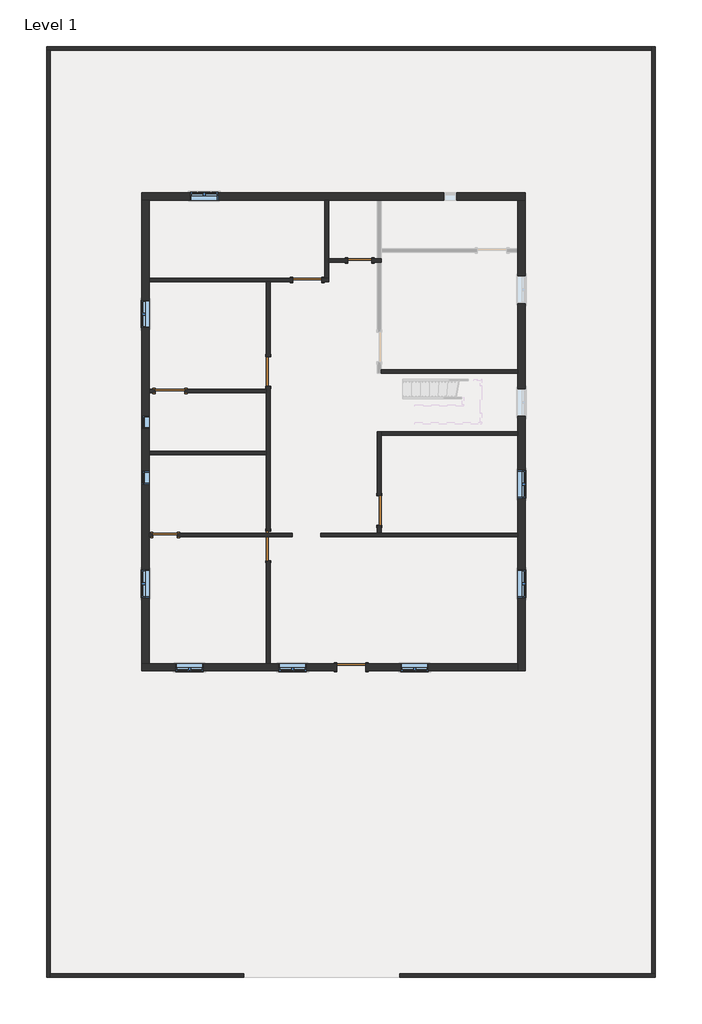
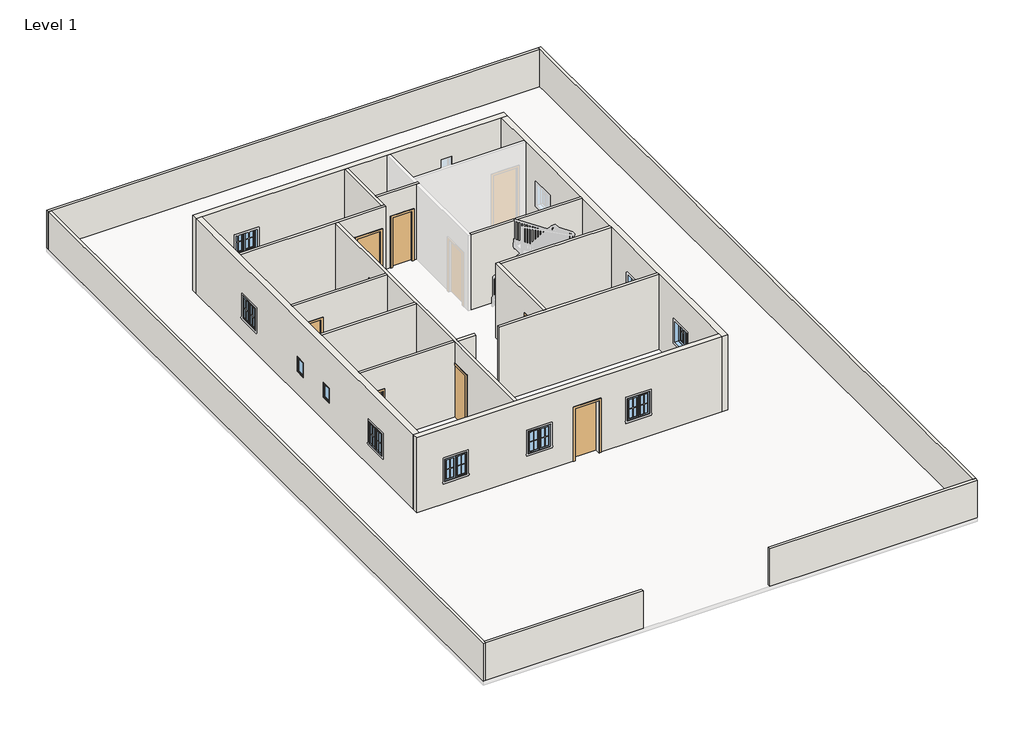
# One storey, part 1 of 3: 20 walls, 10 windows, 8 doors.
"""IFC4 building model written with IfcOpenShell, lengths in millimetres."""

from ifc_helpers import new_model, si_unit, frame, origin, origin_with_axes, place, context, project, spatial, polyline, outline, extrude, faceted_brep, transform, mapped, element, save
from components import door_d8f5dbb5, door_f2b275c1, door_e5f9f3c4, door_305aa2a5, door_a90ba1ad, window_aa618e30, window_339605e1

model = new_model("IFC4")

# Units and contexts
model_context = context("Model", 3, world=origin())
ifc_project = project(units=[si_unit("LENGTHUNIT", "METRE", prefix="MILLI")], contexts=[model_context])

# Site, building, storey
site = spatial("IfcSite", under=ifc_project)
building = spatial("IfcBuilding", under=site)
storey = spatial("IfcBuildingStorey", under=building, Name="Level 1", Elevation=0.0)

# Doors
placement = place(None, origin())
door_shape = door_d8f5dbb5(model_context)
element("IfcDoor", 1, ObjectType="Single-Flush : 30\" x 80\"", at=placement, inside=storey, context=model_context, shape_type="MappedRepresentation", body=[
    mapped(door_shape, transform((-509.1743007, 6967.427558, 0.0), x_axis=(1.0, 0.0, 0.0), y_axis=(0.0, 1.0, 0.0), z_axis=(0.0, 0.0, 1.0))),
])
door_2_shape = door_f2b275c1(model_context)
element("IfcDoor", 2, ObjectType="Single-Flush : 30\" x 80\"", at=placement, inside=storey, context=model_context, shape_type="MappedRepresentation", body=[
    mapped(door_2_shape, transform((-6586.1243007, -1605.072442, 0.0), x_axis=(-1.0, 0.0, 0.0), y_axis=(0.0, -1.0, 0.0), z_axis=(0.0, 0.0, 1.0))),
])
door_3_shape = door_e5f9f3c4(model_context)
element("IfcDoor", 3, ObjectType="Single-Flush : 36\" x 84\"", at=placement, inside=storey, context=model_context, shape_type="MappedRepresentation", body=[
    mapped(door_3_shape, transform((-2147.4743007, 6357.827558, 0.0), x_axis=(1.0, 0.0, 0.0), y_axis=(0.0, 1.0, 0.0), z_axis=(0.0, 0.0, 1.0))),
])
element("IfcDoor", 4, ObjectType="Single-Flush : 36\" x 84\"", at=placement, inside=storey, context=model_context, shape_type="MappedRepresentation", body=[
    mapped(door_3_shape, transform((100.4256993, -843.072442, 0.0), x_axis=(0.0, -1.0, 0.0), y_axis=(1.0, 0.0, 0.0), z_axis=(0.0, 0.0, 1.0))),
])
element("IfcDoor", 5, ObjectType="Single-Flush : 36\" x 84\"", at=placement, inside=storey, context=model_context, shape_type="MappedRepresentation", body=[
    mapped(door_3_shape, transform((-3366.6743007, -1947.972442, 0.0), x_axis=(0.0, 1.0, 0.0), y_axis=(-1.0, 0.0, 0.0), z_axis=(0.0, 0.0, 1.0))),
])
door_4_shape = door_305aa2a5(model_context)
element("IfcDoor", 6, ObjectType="Single-Flush : 36\" x 84\"", at=placement, inside=storey, context=model_context, shape_type="MappedRepresentation", body=[
    mapped(door_4_shape, transform((-6433.7243007, 2890.727558, 0.0), x_axis=(-1.0, 0.0, 0.0), y_axis=(0.0, -1.0, 0.0), z_axis=(0.0, 0.0, 1.0))),
])
element("IfcDoor", 7, ObjectType="Single-Flush : 36\" x 84\"", at=placement, inside=storey, context=model_context, shape_type="MappedRepresentation", body=[
    mapped(door_4_shape, transform((-3366.6743007, 3500.327558, 0.0), x_axis=(0.0, -1.0, 0.0), y_axis=(1.0, 0.0, 0.0), z_axis=(0.0, 0.0, 1.0))),
])
door_5_shape = door_a90ba1ad(model_context)
element("IfcDoor", 8, ObjectType="Single-Flush : 36\" x 84\"", at=placement, inside=storey, context=model_context, shape_type="MappedRepresentation", body=[
    mapped(door_5_shape, transform((-775.8743007, -5738.922442, 0.0), x_axis=(-1.0, 0.0, 0.0), y_axis=(0.0, -1.0, 0.0), z_axis=(0.0, 0.0, 1.0))),
])

# Walls
element("IfcWall", 9, ObjectType="WALL4.5\"", at=placement, inside=storey, context=model_context, shape_type="Brep", body=[
    faceted_brep([(-1690.2743007, 6300.677558, 2133.6), (-1690.2743007, 6300.677558, 0.0), (-1480.7243007, 6300.677558, 0.0), (-1480.7243007, 6300.677558, 3048.0), (-3309.5243007, 6300.677558, 3048.0), (-3423.8243007, 6300.677558, 3048.0), (-7081.4243007, 6300.677558, 3048.0), (-7081.4243007, 6300.677558, 0.0), (-3423.8243007, 6300.677558, 0.0), (-3309.5243007, 6300.677558, 0.0), (-2604.6743007, 6300.677558, 0.0), (-2604.6743007, 6300.677558, 2133.6), (-1480.7243007, 6414.977558, 0.0), (-1595.0243007, 6414.977558, 0.0), (-1690.2743007, 6414.977558, 0.0), (-1690.2743007, 6414.977558, 2133.6), (-2604.6743007, 6414.977558, 2133.6), (-2604.6743007, 6414.977558, 0.0), (-7081.4243007, 6414.977558, 0.0), (-7081.4243007, 6414.977558, 3048.0), (-1595.0243007, 6414.977558, 3048.0), (-1480.7243007, 6414.977558, 3048.0)], [[[0, 1, 2, 3, 4, 5, 6, 7, 8, 9, 10, 11]], [[12, 13, 14, 15, 16, 17, 18, 19, 20, 21]], [[2, 1, 14, 13, 12]], [[10, 9, 8, 7, 18, 17]], [[7, 6, 19, 18]], [[3, 2, 12, 21]], [[15, 14, 1, 0]], [[16, 15, 0, 11]], [[17, 16, 11, 10]], [[6, 5, 4, 3, 21, 20, 19]]]),
])
element("IfcWall", 10, ObjectType="WALL4.5\"", at=placement, inside=storey, context=model_context, shape_type="Brep", body=[
    faceted_brep([(-1480.7243007, 6414.977558, 0.0), (-1480.7243007, 6910.277558, 0.0), (-1480.7243007, 7024.577558, 0.0), (-1480.7243007, 8853.377558, 0.0), (-1480.7243007, 8853.377558, 3048.0), (-1480.7243007, 7024.577558, 3048.0), (-1480.7243007, 6910.277558, 3048.0), (-1480.7243007, 6414.977558, 3048.0), (-1595.0243007, 6414.977558, 0.0), (-1595.0243007, 6414.977558, 3048.0), (-1595.0243007, 8853.377558, 3048.0), (-1595.0243007, 8853.377558, 0.0)], [[[0, 1, 2, 3, 4, 5, 6, 7]], [[8, 9, 10, 11]], [[3, 2, 1, 0, 8, 11]], [[0, 7, 9, 8]], [[4, 3, 11, 10]], [[7, 6, 5, 4, 10, 9]]]),
])
element("IfcWall", 11, ObjectType="WALL4.5\"", at=placement, inside=storey, context=model_context, shape_type="Brep", body=[
    faceted_brep([(-128.1743007, 6910.277558, 2032.0), (-128.1743007, 6910.277558, 0.0), (43.2756993, 6910.277558, 0.0), (157.5756993, 6910.277558, 0.0), (157.5756993, 6910.277558, 3048.0), (43.2756993, 6910.277558, 3048.0), (-1480.7243007, 6910.277558, 3048.0), (-1480.7243007, 6910.277558, 0.0), (-890.1743007, 6910.277558, 0.0), (-890.1743007, 6910.277558, 2032.0), (157.5756993, 7024.577558, 0.0), (43.2756993, 7024.577558, 0.0), (-128.1743007, 7024.577558, 0.0), (-128.1743007, 7024.577558, 2032.0), (-890.1743007, 7024.577558, 2032.0), (-890.1743007, 7024.577558, 0.0), (-1480.7243007, 7024.577558, 0.0), (-1480.7243007, 7024.577558, 3048.0), (43.2756993, 7024.577558, 3048.0), (157.5756993, 7024.577558, 3048.0)], [[[0, 1, 2, 3, 4, 5, 6, 7, 8, 9]], [[10, 11, 12, 13, 14, 15, 16, 17, 18, 19]], [[8, 7, 16, 15]], [[3, 2, 1, 12, 11, 10]], [[7, 6, 17, 16]], [[4, 3, 10, 19]], [[13, 12, 1, 0]], [[14, 13, 0, 9]], [[15, 14, 9, 8]], [[6, 5, 4, 19, 18, 17]]]),
])
element("IfcWall", 12, ObjectType="WALL4.5\"", at=placement, inside=storey, context=model_context, shape_type="Brep", body=[
    faceted_brep([(-3423.8243007, 3043.127558, 0.0), (-3423.8243007, 2947.877558, 0.0), (-3423.8243007, 2833.577558, 0.0), (-3423.8243007, 1004.777558, 0.0), (-3423.8243007, 890.477558, 0.0), (-3423.8243007, -1490.772442, 0.0), (-3423.8243007, -1490.772442, 2133.6), (-3423.8243007, -1547.922442, 2133.6), (-3423.8243007, -1662.222442, 2133.6), (-3423.8243007, -2405.172442, 2133.6), (-3423.8243007, -2405.172442, 0.0), (-3423.8243007, -5624.622442, 0.0), (-3423.8243007, -5624.622442, 3048.0), (-3423.8243007, -1662.222442, 3048.0), (-3423.8243007, -1547.922442, 3048.0), (-3423.8243007, 890.477558, 3048.0), (-3423.8243007, 1004.777558, 3048.0), (-3423.8243007, 2833.577558, 3048.0), (-3423.8243007, 2947.877558, 3048.0), (-3423.8243007, 6300.677558, 3048.0), (-3423.8243007, 6300.677558, 0.0), (-3423.8243007, 3957.527558, 0.0), (-3423.8243007, 3957.527558, 2133.6), (-3423.8243007, 3043.127558, 2133.6), (-3309.5243007, -1490.772442, 2133.6), (-3309.5243007, -1490.772442, 0.0), (-3309.5243007, 3043.127558, 0.0), (-3309.5243007, 3043.127558, 2133.6), (-3309.5243007, 3957.527558, 2133.6), (-3309.5243007, 3957.527558, 0.0), (-3309.5243007, 6300.677558, 0.0), (-3309.5243007, 6300.677558, 3048.0), (-3309.5243007, -1547.922442, 3048.0), (-3309.5243007, -1662.222442, 3048.0), (-3309.5243007, -5624.622442, 3048.0), (-3309.5243007, -5624.622442, 0.0), (-3309.5243007, -2405.172442, 0.0), (-3309.5243007, -2405.172442, 2133.6), (-3309.5243007, -1662.222442, 2133.6), (-3309.5243007, -1547.922442, 2133.6)], [[[0, 1, 2, 3, 4, 5, 6, 7, 8, 9, 10, 11, 12, 13, 14, 15, 16, 17, 18, 19, 20, 21, 22, 23]], [[24, 25, 26, 27, 28, 29, 30, 31, 32, 33, 34, 35, 36, 37, 38, 39]], [[21, 20, 30, 29]], [[36, 35, 11, 10]], [[26, 25, 5, 4, 3, 2, 1, 0]], [[12, 11, 35, 34]], [[20, 19, 31, 30]], [[27, 26, 0, 23]], [[28, 27, 23, 22]], [[29, 28, 22, 21]], [[6, 5, 25, 24]], [[9, 8, 7, 6, 24, 39, 38, 37]], [[10, 9, 37, 36]], [[19, 18, 17, 16, 15, 14, 13, 12, 34, 33, 32, 31]]]),
])
element("IfcWall", 13, ObjectType="WALL4.5\"", at=placement, inside=storey, context=model_context, shape_type="Brep", body=[
    faceted_brep([(157.5756993, -1547.922442, 0.0), (157.5756993, -1300.272442, 0.0), (157.5756993, -1300.272442, 2133.6), (157.5756993, -385.872442, 2133.6), (157.5756993, -385.872442, 0.0), (157.5756993, 1500.077558, 0.0), (157.5756993, 1614.377558, 0.0), (157.5756993, 1614.377558, 3048.0), (157.5756993, 1500.077558, 3048.0), (157.5756993, -1547.922442, 3048.0), (43.2756993, -1300.272442, 2133.6), (43.2756993, -1300.272442, 0.0), (43.2756993, -1547.922442, 0.0), (43.2756993, -1547.922442, 3048.0), (43.2756993, 1614.377558, 3048.0), (43.2756993, 1614.377558, 0.0), (43.2756993, -385.872442, 0.0), (43.2756993, -385.872442, 2133.6)], [[[0, 1, 2, 3, 4, 5, 6, 7, 8, 9]], [[10, 11, 12, 13, 14, 15, 16, 17]], [[16, 15, 6, 5, 4]], [[12, 11, 1, 0]], [[7, 6, 15, 14]], [[0, 9, 13, 12]], [[2, 1, 11, 10]], [[3, 2, 10, 17]], [[4, 3, 17, 16]], [[9, 8, 7, 14, 13]]]),
])
element("IfcWall", 14, ObjectType="WALL4.5\"", at=placement, inside=storey, context=model_context, shape_type="SweptSolid", body=[
    extrude(outline(polyline([(4424.7756993, 1500.077558), (157.5756993, 1500.077558), (157.5756993, 1614.377558), (4424.7756993, 1614.377558), (4424.7756993, 1500.077558)])), origin_with_axes(), (0.0, 0.0, 1.0), 3048.0),
])
element("IfcWall", 15, ObjectType="WALL4.5\"", at=placement, inside=storey, context=model_context, shape_type="SweptSolid", body=[
    extrude(outline(polyline([(-3423.8243007, 890.477558), (-7081.4243007, 890.477558), (-7081.4243007, 1004.777558), (-3423.8243007, 1004.777558), (-3423.8243007, 890.477558)])), origin_with_axes(), (0.0, 0.0, 1.0), 3048.0),
])
element("IfcWall", 16, ObjectType="WALL4.5\"", at=placement, inside=storey, context=model_context, shape_type="SweptSolid", body=[
    extrude(outline(polyline([(0.0, -7081.4243007), (0.0, -6890.9243007), (2133.6, -6890.9243007), (2133.6, -5976.5243007), (0.0, -5976.5243007), (0.0, -3423.8243007), (3048.0, -3423.8243007), (3048.0, -7081.4243007), (0.0, -7081.4243007)])), frame((0.0, 2833.577558, 0.0), z_axis=(0.0, 1.0, 0.0), x_axis=(0.0, 0.0, 1.0)), (0.0, 0.0, 1.0), 114.3),
])
element("IfcWall", 17, ObjectType="WALL4.5\"", at=placement, inside=storey, context=model_context, shape_type="SweptSolid", body=[
    extrude(outline(polyline([(4424.7756993, 3443.177558), (157.5756993, 3443.177558), (157.5756993, 3557.477558), (4424.7756993, 3557.477558), (4424.7756993, 3443.177558)])), origin_with_axes(), (0.0, 0.0, 1.0), 3048.0),
])
element("IfcWall", 18, ObjectType="WALL4.5\"", at=placement, inside=storey, context=model_context, shape_type="SweptSolid", body=[
    extrude(outline(polyline([(0.0, -2614.8628774), (3048.0, -2614.8628774), (3048.0, -3309.5243007), (2133.6, -3309.5243007), (2133.6, -3423.8243007), (3048.0, -3423.8243007), (3048.0, -7081.4243007), (0.0, -7081.4243007), (0.0, -6967.1243007), (2032.0, -6967.1243007), (2032.0, -6205.1243007), (0.0, -6205.1243007), (0.0, -2614.8628774)])), frame((0.0, -1662.222442, 0.0), z_axis=(0.0, 1.0, 0.0), x_axis=(0.0, 0.0, 1.0)), (0.0, 0.0, 1.0), 114.3),
])
element("IfcWall", 19, ObjectType="WALL4.5\"", at=placement, inside=storey, context=model_context, shape_type="Brep", body=[
    faceted_brep([(-1720.6441625, -1662.222442, 0.0), (4424.7756993, -1662.222442, 0.0), (4424.7756993, -1662.222442, 3048.0), (-1720.6441625, -1662.222442, 3048.0), (-1720.6441625, -1547.922442, 0.0), (-1720.6441625, -1547.922442, 3048.0), (43.2756993, -1547.922442, 3048.0), (157.5756993, -1547.922442, 3048.0), (4424.7756993, -1547.922442, 3048.0), (4424.7756993, -1547.922442, 0.0), (157.5756993, -1547.922442, 0.0), (43.2756993, -1547.922442, 0.0)], [[[0, 1, 2, 3]], [[4, 5, 6, 7, 8, 9, 10, 11]], [[1, 0, 4, 11, 10, 9]], [[0, 3, 5, 4]], [[2, 1, 9, 8]], [[3, 2, 8, 7, 6, 5]]]),
])
element("IfcWall", 20, ObjectType="WALL4.5\"", at=placement, inside=storey, context=model_context, shape_type="Brep", body=[
    faceted_brep([(-10290.3086707, 13531.2370172, 0.0), (-10176.0086707, 13531.2370172, 0.0), (8607.2913293, 13531.2370172, 0.0), (8607.2913293, 13531.2370172, 1524.0), (-10176.0086707, 13531.2370172, 1524.0), (-10290.3086707, 13531.2370172, 1524.0), (-10290.3086707, 13645.5370172, 0.0), (-10290.3086707, 13645.5370172, 1524.0), (8607.2913293, 13645.5370172, 1524.0), (8607.2913293, 13645.5370172, 0.0)], [[[0, 1, 2, 3, 4, 5]], [[6, 7, 8, 9]], [[2, 1, 0, 6, 9]], [[5, 4, 3, 8, 7]], [[0, 5, 7, 6]], [[3, 2, 9, 8]]]),
])
element("IfcWall", 21, ObjectType="WALL4.5\"", at=placement, inside=storey, context=model_context, shape_type="Brep", body=[
    faceted_brep([(-10176.0086707, -15424.7629828, 0.0), (-10176.0086707, -15310.4629828, 0.0), (-10176.0086707, 13531.2370172, 0.0), (-10176.0086707, 13531.2370172, 1524.0), (-10176.0086707, -15310.4629828, 1524.0), (-10176.0086707, -15424.7629828, 1524.0), (-10290.3086707, -15424.7629828, 0.0), (-10290.3086707, -15424.7629828, 1524.0), (-10290.3086707, 13531.2370172, 1524.0), (-10290.3086707, 13531.2370172, 0.0)], [[[0, 1, 2, 3, 4, 5]], [[6, 7, 8, 9]], [[2, 1, 0, 6, 9]], [[5, 4, 3, 8, 7]], [[0, 5, 7, 6]], [[3, 2, 9, 8]]]),
])
element("IfcWall", 22, ObjectType="WALL4.5\"", at=placement, inside=storey, context=model_context, shape_type="Brep", body=[
    faceted_brep([(8721.5913293, -15310.4629828, 0.0), (8607.2913293, -15310.4629828, 0.0), (739.6413293, -15310.4629828, 0.0), (739.6413293, -15310.4629828, 1524.0), (8607.2913293, -15310.4629828, 1524.0), (8721.5913293, -15310.4629828, 1524.0), (8721.5913293, -15424.7629828, 0.0), (8721.5913293, -15424.7629828, 1524.0), (739.6413293, -15424.7629828, 1524.0), (739.6413293, -15424.7629828, 0.0)], [[[0, 1, 2, 3, 4, 5]], [[6, 7, 8, 9]], [[2, 1, 0, 6, 9]], [[3, 2, 9, 8]], [[5, 4, 3, 8, 7]], [[0, 5, 7, 6]]]),
])
element("IfcWall", 23, ObjectType="WALL4.5\"", at=placement, inside=storey, context=model_context, shape_type="Brep", body=[
    faceted_brep([(8607.2913293, 13645.5370172, 0.0), (8607.2913293, 13531.2370172, 0.0), (8607.2913293, -15310.4629828, 0.0), (8607.2913293, -15310.4629828, 1524.0), (8607.2913293, 13531.2370172, 1524.0), (8607.2913293, 13645.5370172, 1524.0), (8721.5913293, 13645.5370172, 0.0), (8721.5913293, 13645.5370172, 1524.0), (8721.5913293, -15310.4629828, 1524.0), (8721.5913293, -15310.4629828, 0.0)], [[[0, 1, 2, 3, 4, 5]], [[6, 7, 8, 9]], [[2, 1, 0, 6, 9]], [[5, 4, 3, 8, 7]], [[0, 5, 7, 6]], [[3, 2, 9, 8]]]),
])
element("IfcWall", 24, ObjectType="WALL4.5\"", at=placement, inside=storey, context=model_context, shape_type="SweptSolid", body=[
    extrude(outline(polyline([(-10176.0086707, -15310.4629828), (-4137.1586707, -15310.4629828), (-4137.1586707, -15424.7629828), (-10176.0086707, -15424.7629828), (-10176.0086707, -15310.4629828)])), origin_with_axes(), (0.0, 0.0, 1.0), 1524.0),
])
element("IfcWall", 25, ObjectType="WALL9\"", at=placement, inside=storey, context=model_context, shape_type="Brep", body=[
    faceted_brep([(-7310.0243007, 8853.377558, 0.0), (-7081.4243007, 8853.377558, 0.0), (-1595.0243007, 8853.377558, 0.0), (-1480.7243007, 8853.377558, 0.0), (43.2756993, 8853.377558, 0.0), (157.5756993, 8853.377558, 0.0), (4424.7756993, 8853.377558, 0.0), (4653.3756993, 8853.377558, 0.0), (4653.3756993, 8853.377558, 3048.0), (4424.7756993, 8853.377558, 3048.0), (157.5756993, 8853.377558, 3048.0), (43.2756993, 8853.377558, 3048.0), (-1480.7243007, 8853.377558, 3048.0), (-1595.0243007, 8853.377558, 3048.0), (-7081.4243007, 8853.377558, 3048.0), (-7310.0243007, 8853.377558, 3048.0), (-4935.1243007, 8853.377558, 1828.8), (-4935.1243007, 8853.377558, 914.4), (-5798.7243007, 8853.377558, 914.4), (-5798.7243007, 8853.377558, 1828.8), (2522.9506993, 8853.377558, 2133.6), (2522.9506993, 8853.377558, 304.8), (2116.5506993, 8853.377558, 304.8), (2116.5506993, 8853.377558, 2133.6), (-7310.0243007, 9081.977558, 0.0), (-7310.0243007, 9081.977558, 3048.0), (4653.3756993, 9081.977558, 3048.0), (4653.3756993, 9081.977558, 0.0), (-4935.1243007, 9081.977558, 1828.8), (-5798.7243007, 9081.977558, 1828.8), (-5798.7243007, 9081.977558, 914.4), (-4935.1243007, 9081.977558, 914.4), (2522.9506993, 9081.977558, 2133.6), (2116.5506993, 9081.977558, 2133.6), (2116.5506993, 9081.977558, 304.8), (2522.9506993, 9081.977558, 304.8)], [[[0, 1, 2, 3, 4, 5, 6, 7, 8, 9, 10, 11, 12, 13, 14, 15], [16, 17, 18, 19], [20, 21, 22, 23]], [[24, 25, 26, 27], [28, 29, 30, 31], [32, 33, 34, 35]], [[7, 6, 5, 4, 3, 2, 1, 0, 24, 27]], [[8, 7, 27, 26]], [[0, 15, 25, 24]], [[17, 16, 28, 31]], [[18, 17, 31, 30]], [[19, 18, 30, 29]], [[16, 19, 29, 28]], [[21, 20, 32, 35]], [[22, 21, 35, 34]], [[23, 22, 34, 33]], [[20, 23, 33, 32]], [[15, 14, 13, 12, 11, 10, 9, 8, 26, 25]]]),
])
element("IfcWall", 26, ObjectType="WALL9\"", at=placement, inside=storey, context=model_context, shape_type="Brep", body=[
    faceted_brep([(4424.7756993, 8853.377558, 0.0), (4424.7756993, 7329.377558, 0.0), (4424.7756993, 7215.077558, 0.0), (4424.7756993, 3557.477558, 0.0), (4424.7756993, 3443.177558, 0.0), (4424.7756993, 1614.377558, 0.0), (4424.7756993, 1500.077558, 0.0), (4424.7756993, -1547.922442, 0.0), (4424.7756993, -1662.222442, 0.0), (4424.7756993, -5624.622442, 0.0), (4424.7756993, -5853.222442, 0.0), (4424.7756993, -5853.222442, 3048.0), (4424.7756993, -5624.622442, 3048.0), (4424.7756993, -1662.222442, 3048.0), (4424.7756993, -1547.922442, 3048.0), (4424.7756993, 1500.077558, 3048.0), (4424.7756993, 1614.377558, 3048.0), (4424.7756993, 3443.177558, 3048.0), (4424.7756993, 3557.477558, 3048.0), (4424.7756993, 7215.077558, 3048.0), (4424.7756993, 7329.377558, 3048.0), (4424.7756993, 8853.377558, 3048.0), (4424.7756993, 5621.227558, 1828.8), (4424.7756993, 5621.227558, 914.4), (4424.7756993, 6484.827558, 914.4), (4424.7756993, 6484.827558, 1828.8), (4424.7756993, 2096.977558, 1828.8), (4424.7756993, 2096.977558, 914.4), (4424.7756993, 2960.577558, 914.4), (4424.7756993, 2960.577558, 1828.8), (4424.7756993, -455.722442, 1828.8), (4424.7756993, -455.722442, 914.4), (4424.7756993, 407.877558, 914.4), (4424.7756993, 407.877558, 1828.8), (4424.7756993, -3560.872442, 1828.8), (4424.7756993, -3560.872442, 914.4), (4424.7756993, -2697.272442, 914.4), (4424.7756993, -2697.272442, 1828.8), (4653.3756993, 8853.377558, 0.0), (4653.3756993, 8853.377558, 3048.0), (4653.3756993, -5853.222442, 3048.0), (4653.3756993, -5853.222442, 0.0), (4653.3756993, 5621.227558, 1828.8), (4653.3756993, 6484.827558, 1828.8), (4653.3756993, 6484.827558, 914.4), (4653.3756993, 5621.227558, 914.4), (4653.3756993, 2096.977558, 1828.8), (4653.3756993, 2960.577558, 1828.8), (4653.3756993, 2960.577558, 914.4), (4653.3756993, 2096.977558, 914.4), (4653.3756993, -455.722442, 1828.8), (4653.3756993, 407.877558, 1828.8), (4653.3756993, 407.877558, 914.4), (4653.3756993, -455.722442, 914.4), (4653.3756993, -3560.872442, 1828.8), (4653.3756993, -2697.272442, 1828.8), (4653.3756993, -2697.272442, 914.4), (4653.3756993, -3560.872442, 914.4)], [[[0, 1, 2, 3, 4, 5, 6, 7, 8, 9, 10, 11, 12, 13, 14, 15, 16, 17, 18, 19, 20, 21], [22, 23, 24, 25], [26, 27, 28, 29], [30, 31, 32, 33], [34, 35, 36, 37]], [[38, 39, 40, 41], [42, 43, 44, 45], [46, 47, 48, 49], [50, 51, 52, 53], [54, 55, 56, 57]], [[10, 9, 8, 7, 6, 5, 4, 3, 2, 1, 0, 38, 41]], [[0, 21, 39, 38]], [[11, 10, 41, 40]], [[23, 22, 42, 45]], [[24, 23, 45, 44]], [[25, 24, 44, 43]], [[22, 25, 43, 42]], [[27, 26, 46, 49]], [[28, 27, 49, 48]], [[29, 28, 48, 47]], [[26, 29, 47, 46]], [[31, 30, 50, 53]], [[32, 31, 53, 52]], [[33, 32, 52, 51]], [[30, 33, 51, 50]], [[35, 34, 54, 57]], [[36, 35, 57, 56]], [[37, 36, 56, 55]], [[34, 37, 55, 54]], [[21, 20, 19, 18, 17, 16, 15, 14, 13, 12, 11, 40, 39]]]),
])
element("IfcWall", 27, ObjectType="WALL9\"", at=placement, inside=storey, context=model_context, shape_type="Brep", body=[
    faceted_brep([(-1233.0743007, -5624.622442, 2133.6), (-1233.0743007, -5624.622442, 0.0), (-3309.5243007, -5624.622442, 0.0), (-3423.8243007, -5624.622442, 0.0), (-7081.4243007, -5624.622442, 0.0), (-7310.0243007, -5624.622442, 0.0), (-7310.0243007, -5624.622442, 3048.0), (-7081.4243007, -5624.622442, 3048.0), (-3423.8243007, -5624.622442, 3048.0), (-3309.5243007, -5624.622442, 3048.0), (4424.7756993, -5624.622442, 3048.0), (4424.7756993, -5624.622442, 0.0), (-318.6743007, -5624.622442, 0.0), (-318.6743007, -5624.622442, 2133.6), (773.5256993, -5624.622442, 1828.8), (773.5256993, -5624.622442, 914.4), (1637.1256993, -5624.622442, 914.4), (1637.1256993, -5624.622442, 1828.8), (-3036.4743007, -5624.622442, 1828.8), (-3036.4743007, -5624.622442, 914.4), (-2172.8743007, -5624.622442, 914.4), (-2172.8743007, -5624.622442, 1828.8), (-6255.9243007, -5624.622442, 1828.8), (-6255.9243007, -5624.622442, 914.4), (-5392.3243007, -5624.622442, 914.4), (-5392.3243007, -5624.622442, 1828.8), (-7310.0243007, -5853.222442, 0.0), (-1233.0743007, -5853.222442, 0.0), (-1233.0743007, -5853.222442, 2133.6), (-318.6743007, -5853.222442, 2133.6), (-318.6743007, -5853.222442, 0.0), (4424.7756993, -5853.222442, 0.0), (4424.7756993, -5853.222442, 3048.0), (-7310.0243007, -5853.222442, 3048.0), (773.5256993, -5853.222442, 1828.8), (1637.1256993, -5853.222442, 1828.8), (1637.1256993, -5853.222442, 914.4), (773.5256993, -5853.222442, 914.4), (-3036.4743007, -5853.222442, 1828.8), (-2172.8743007, -5853.222442, 1828.8), (-2172.8743007, -5853.222442, 914.4), (-3036.4743007, -5853.222442, 914.4), (-6255.9243007, -5853.222442, 1828.8), (-5392.3243007, -5853.222442, 1828.8), (-5392.3243007, -5853.222442, 914.4), (-6255.9243007, -5853.222442, 914.4)], [[[0, 1, 2, 3, 4, 5, 6, 7, 8, 9, 10, 11, 12, 13], [14, 15, 16, 17], [18, 19, 20, 21], [22, 23, 24, 25]], [[26, 27, 28, 29, 30, 31, 32, 33], [34, 35, 36, 37], [38, 39, 40, 41], [42, 43, 44, 45]], [[12, 11, 31, 30]], [[5, 4, 3, 2, 1, 27, 26]], [[11, 10, 32, 31]], [[6, 5, 26, 33]], [[28, 27, 1, 0]], [[29, 28, 0, 13]], [[30, 29, 13, 12]], [[15, 14, 34, 37]], [[16, 15, 37, 36]], [[17, 16, 36, 35]], [[14, 17, 35, 34]], [[19, 18, 38, 41]], [[20, 19, 41, 40]], [[21, 20, 40, 39]], [[18, 21, 39, 38]], [[23, 22, 42, 45]], [[24, 23, 45, 44]], [[25, 24, 44, 43]], [[22, 25, 43, 42]], [[10, 9, 8, 7, 6, 33, 32]]]),
])
element("IfcWall", 28, ObjectType="WALL9\"", at=placement, inside=storey, context=model_context, shape_type="Brep", body=[
    faceted_brep([(-7081.4243007, -5624.622442, 0.0), (-7081.4243007, -1662.222442, 0.0), (-7081.4243007, -1547.922442, 0.0), (-7081.4243007, 890.477558, 0.0), (-7081.4243007, 1004.777558, 0.0), (-7081.4243007, 2833.577558, 0.0), (-7081.4243007, 2947.877558, 0.0), (-7081.4243007, 6300.677558, 0.0), (-7081.4243007, 6414.977558, 0.0), (-7081.4243007, 8853.377558, 0.0), (-7081.4243007, 8853.377558, 3048.0), (-7081.4243007, 6414.977558, 3048.0), (-7081.4243007, 6300.677558, 3048.0), (-7081.4243007, 2947.877558, 3048.0), (-7081.4243007, 2833.577558, 3048.0), (-7081.4243007, 1004.777558, 3048.0), (-7081.4243007, 890.477558, 3048.0), (-7081.4243007, -1547.922442, 3048.0), (-7081.4243007, -1662.222442, 3048.0), (-7081.4243007, -5624.622442, 3048.0), (-7081.4243007, 388.827558, 1524.0), (-7081.4243007, 388.827558, 914.4), (-7081.4243007, -17.572442, 914.4), (-7081.4243007, -17.572442, 1524.0), (-7081.4243007, 2122.377558, 1524.0), (-7081.4243007, 2122.377558, 914.4), (-7081.4243007, 1715.977558, 914.4), (-7081.4243007, 1715.977558, 1524.0), (-7081.4243007, 5722.827558, 1828.8), (-7081.4243007, 5722.827558, 914.4), (-7081.4243007, 4859.227558, 914.4), (-7081.4243007, 4859.227558, 1828.8), (-7081.4243007, -2697.272442, 1828.8), (-7081.4243007, -2697.272442, 914.4), (-7081.4243007, -3560.872442, 914.4), (-7081.4243007, -3560.872442, 1828.8), (-7310.0243007, -5624.622442, 0.0), (-7310.0243007, -5624.622442, 3048.0), (-7310.0243007, 8853.377558, 3048.0), (-7310.0243007, 8853.377558, 0.0), (-7310.0243007, 388.827558, 1524.0), (-7310.0243007, -17.572442, 1524.0), (-7310.0243007, -17.572442, 914.4), (-7310.0243007, 388.827558, 914.4), (-7310.0243007, 2122.377558, 1524.0), (-7310.0243007, 1715.977558, 1524.0), (-7310.0243007, 1715.977558, 914.4), (-7310.0243007, 2122.377558, 914.4), (-7310.0243007, 5722.827558, 1828.8), (-7310.0243007, 4859.227558, 1828.8), (-7310.0243007, 4859.227558, 914.4), (-7310.0243007, 5722.827558, 914.4), (-7310.0243007, -2697.272442, 1828.8), (-7310.0243007, -3560.872442, 1828.8), (-7310.0243007, -3560.872442, 914.4), (-7310.0243007, -2697.272442, 914.4)], [[[0, 1, 2, 3, 4, 5, 6, 7, 8, 9, 10, 11, 12, 13, 14, 15, 16, 17, 18, 19], [20, 21, 22, 23], [24, 25, 26, 27], [28, 29, 30, 31], [32, 33, 34, 35]], [[36, 37, 38, 39], [40, 41, 42, 43], [44, 45, 46, 47], [48, 49, 50, 51], [52, 53, 54, 55]], [[9, 8, 7, 6, 5, 4, 3, 2, 1, 0, 36, 39]], [[10, 9, 39, 38]], [[0, 19, 37, 36]], [[21, 20, 40, 43]], [[22, 21, 43, 42]], [[23, 22, 42, 41]], [[20, 23, 41, 40]], [[25, 24, 44, 47]], [[26, 25, 47, 46]], [[27, 26, 46, 45]], [[24, 27, 45, 44]], [[29, 28, 48, 51]], [[30, 29, 51, 50]], [[31, 30, 50, 49]], [[28, 31, 49, 48]], [[33, 32, 52, 55]], [[34, 33, 55, 54]], [[35, 34, 54, 53]], [[32, 35, 53, 52]], [[19, 18, 17, 16, 15, 14, 13, 12, 11, 10, 38, 37]]]),
])

# Windows
window_shape = window_aa618e30(model_context)
element("IfcWindow", 29, ObjectType="Fixed : 16\" x 24\"", at=placement, inside=storey, context=model_context, shape_type="MappedRepresentation", body=[
    mapped(window_shape, transform((-7195.7243007, 223.727558, 0.0), x_axis=(0.0, 1.0, 0.0), y_axis=(-1.0, 0.0, 0.0), z_axis=(0.0, 0.0, 1.0))),
])
element("IfcWindow", 30, ObjectType="Fixed : 16\" x 24\"", at=placement, inside=storey, context=model_context, shape_type="MappedRepresentation", body=[
    mapped(window_shape, transform((-7195.7243007, 1957.277558, 0.0), x_axis=(0.0, 1.0, 0.0), y_axis=(-1.0, 0.0, 0.0), z_axis=(0.0, 0.0, 1.0))),
])
window_2_shape = window_339605e1(model_context)
element("IfcWindow", 31, ObjectType="Window-Casement-Double : 34\" x 36\"", at=placement, inside=storey, context=model_context, shape_type="MappedRepresentation", body=[
    mapped(window_2_shape, transform((-5366.9243007, 8967.677558, 0.0), x_axis=(1.0, 0.0, 0.0), y_axis=(0.0, 1.0, 0.0), z_axis=(0.0, 0.0, 1.0))),
])
element("IfcWindow", 32, ObjectType="Window-Casement-Double : 34\" x 36\"", at=placement, inside=storey, context=model_context, shape_type="MappedRepresentation", body=[
    mapped(window_2_shape, transform((-7195.7243007, 5291.027558, 0.0), x_axis=(0.0, 1.0, 0.0), y_axis=(-1.0, 0.0, 0.0), z_axis=(0.0, 0.0, 1.0))),
])
element("IfcWindow", 33, ObjectType="Window-Casement-Double : 34\" x 36\"", at=placement, inside=storey, context=model_context, shape_type="MappedRepresentation", body=[
    mapped(window_2_shape, transform((4539.0756993, -23.922442, 0.0), x_axis=(0.0, -1.0, 0.0), y_axis=(1.0, 0.0, 0.0), z_axis=(0.0, 0.0, 1.0))),
])
element("IfcWindow", 34, ObjectType="Window-Casement-Double : 34\" x 36\"", at=placement, inside=storey, context=model_context, shape_type="MappedRepresentation", body=[
    mapped(window_2_shape, transform((4539.0756993, -3129.072442, 0.0), x_axis=(0.0, -1.0, 0.0), y_axis=(1.0, 0.0, 0.0), z_axis=(0.0, 0.0, 1.0))),
])
element("IfcWindow", 35, ObjectType="Window-Casement-Double : 34\" x 36\"", at=placement, inside=storey, context=model_context, shape_type="MappedRepresentation", body=[
    mapped(window_2_shape, transform((1205.3256993, -5738.922442, 0.0), x_axis=(-1.0, 0.0, 0.0), y_axis=(0.0, -1.0, 0.0), z_axis=(0.0, 0.0, 1.0))),
])
element("IfcWindow", 36, ObjectType="Window-Casement-Double : 34\" x 36\"", at=placement, inside=storey, context=model_context, shape_type="MappedRepresentation", body=[
    mapped(window_2_shape, transform((-2604.6743007, -5738.922442, 0.0), x_axis=(-1.0, 0.0, 0.0), y_axis=(0.0, -1.0, 0.0), z_axis=(0.0, 0.0, 1.0))),
])
element("IfcWindow", 37, ObjectType="Window-Casement-Double : 34\" x 36\"", at=placement, inside=storey, context=model_context, shape_type="MappedRepresentation", body=[
    mapped(window_2_shape, transform((-5824.1243007, -5738.922442, 0.0), x_axis=(-1.0, 0.0, 0.0), y_axis=(0.0, -1.0, 0.0), z_axis=(0.0, 0.0, 1.0))),
])
element("IfcWindow", 38, ObjectType="Window-Casement-Double : 34\" x 36\"", at=placement, inside=storey, context=model_context, shape_type="MappedRepresentation", body=[
    mapped(window_2_shape, transform((-7195.7243007, -3129.072442, 0.0), x_axis=(0.0, 1.0, 0.0), y_axis=(-1.0, 0.0, 0.0), z_axis=(0.0, 0.0, 1.0))),
])

save(model, "model.ifc")

# Revit data of these elements
# Type "Single-Flush : 30\" x 80\""
#   Type Mark = "5"
#   Construction Type Id = "MDOOR"
#   Assembly Code = "C1020"
#   Analytic Construction = "Metal"
#   Thickness = 0' - 2"
#   Heat Transfer Coefficient (U) = 0.651978 BTU/(h·ft²·°F)
#   Height = 6' - 8"
#   Trim Projection Ext = 0' - 1"
#   Trim Projection Int = 0' - 1"
#   Trim Width = 0' - 3"
#   Width = 2' - 6"
#   Define Thermal Properties by = 1
#   Define Thermal Properties by = 1
#   Door Material = Door - Panel
#   Frame Material = Door - Frame
#   Visual Light Transmittance = 0
#   Solar Heat Gain Coefficient = 0
#   Function = (empty or 0)
#   Wall Closure = (empty or 0)
# Type "Single-Flush : 36\" x 84\""
#   Type Mark = "1"
#   Construction Type Id = "MDOOR"
#   Assembly Code = "C1020"
#   Analytic Construction = "Metal"
#   Thickness = 0' - 2"
#   Heat Transfer Coefficient (U) = 0.651978 BTU/(h·ft²·°F)
#   Height = 7' - 0"
#   Trim Projection Ext = 0' - 1"
#   Trim Projection Int = 0' - 1"
#   Trim Width = 0' - 3"
#   Width = 3' - 0"
#   Define Thermal Properties by = 1
#   Define Thermal Properties by = 1
#   Door Material = Door - Panel
#   Frame Material = Door - Frame
#   Visual Light Transmittance = 0
#   Solar Heat Gain Coefficient = 0
#   Function = (empty or 0)
#   Wall Closure = (empty or 0)
# Type "WALL4.5\""
#   Assembly Code = "B2010"
#   Layers, outside or top first: 0' - 4 1/2" no material (function 1)
# Type "WALL9\""
#   Assembly Code = "B2010"
#   Layers, outside or top first: 0' - 9" no material (function 1)
# Type "Fixed : 16\" x 24\""
#   Type Mark = "4"
#   Construction Type Id = "GSP4R"
#   Assembly Code = "B2020100"
#   Analytic Construction = "1/8 in Pilkington single glazing"
#   Visual Light Transmittance = 0.9
#   Solar Heat Gain Coefficient = 0.78
#   Heat Transfer Coefficient (U) = 0.6496 BTU/(h·ft²·°F)
#   Height = 2' - 0"
#   Default Sill Height = 3' - 0"
#   Width = 1' - 4"
#   Window Inset = 0' - 0 3/4"
#   Define Thermal Properties by = 1
#   Define Thermal Properties by = 1
#   Glass Pane Material = Glass
#   Sash Material = Sash
#   Wall Closure = (empty or 0)
# Type "Window-Casement-Double : 34\" x 36\""
#   Type Mark = "14"
#   Fire Rating = "0.5h"
#   Assembly Code = "B2020100"
#   Analytic Construction = "Double glazing - domestic"
#   Frame Extension [instance default] = 0' - 0 1/4"
#   Window Inset [instance default] = 0' - 0"
#   Wall Thickness [instance default] = 0' - 6"
#   Interior Wall Closure [instance default] = 0' - 2 1/4"
#   Half Width = 1' - 5"
#   Visual Light Transmittance = 0.81
#   Thermal Resistance (R) = 1.8146 (h·ft²·°F)/BTU
#   Solar Heat Gain Coefficient = 0.76
#   Rough Width = 2' - 10 1/2"
#   Rough Height = 3' - 0 1/2"
#   Height = 3' - 0"
#   Heat Transfer Coefficient (U) = 0.5511 BTU/(h·ft²·°F)
#   Exterior Wall Closure [instance default] = 0' - 1 1/4"
#   Extension Jamb [instance default] = 0' - 2 1/4"
#   Default Sill Height = 3' - 0"
#   Width = 2' - 10"
#   Define Thermal Properties by = 0
#   Muntin Visibility = yes
#   Interior Trim Visibility [instance default] = yes
#   Exterior Trim Visibility [instance default] = yes
#   Extension Jamb Visibility [instance default] = yes
#   Interior Trim Material = Wood - Stained
#   Muntin Pattern = Muntin Pattern_2x2 : Muntin Pattern_2x2
#   Interior Trim = Trim-Window-Interior-Flat : Picture Frame
#   Interior Frame Material = Wood - Stained
#   Glass Panel Material = Glass
#   Exterior Trim Material = Clad - White
#   Exterior Trim = Trim-Window-Exterior-Flat : with Sill
#   Exterior Frame Material = Clad - White
#   Wall Closure = (empty or 0)
# Elements 1, 2 (IfcDoor, "Single-Flush : 30\" x 80\"")
#   Phase Created = New Construction
#   Materials on its faces: "Door - Frame", "Door - Panel"
# Elements 3, 4, 5, 6, 7, 8 (IfcDoor, "Single-Flush : 36\" x 84\"")
#   Phase Created = New Construction
#   Materials on its faces: "Door - Frame", "Door - Panel"
# Elements 9, 10, 11, 12, 13, 14, 15, 16, 17, 18, 19 (IfcWall, "WALL4.5\"")
#   Top Offset = 0' - 0"
#   Base Offset = 0' - 0"
#   Unconnected Height = 10' - 0"
#   wall height = 10' - 0"
#   Phase Created = New Construction
#   Base Constraint = Level 1
#   Materials on its faces: "Default Wall"
# Elements 20, 21, 22, 23, 24 (IfcWall, "WALL4.5\"")
#   Top Offset = 0' - 0"
#   Base Offset = 0' - 0"
#   Unconnected Height = 5' - 0"
#   wall height = 5' - 0"
#   Phase Created = New Construction
#   Base Constraint = Level 1
#   Materials on its faces: "Default Wall"
# Elements 25, 26, 27, 28 (IfcWall, "WALL9\"")
#   Top Offset = 0' - 0"
#   Base Offset = 0' - 0"
#   Unconnected Height = 10' - 0"
#   wall height = 10' - 0"
#   Phase Created = New Construction
#   Base Constraint = Level 1
#   Materials on its faces: "Default Wall"
# Element 29 (IfcWindow, "Fixed : 16\" x 24\"")
#   Mark = "2"
#   Phase Created = New Construction
#   Materials on its faces: "Sash", "Glass"
# Element 30 (IfcWindow, "Fixed : 16\" x 24\"")
#   Mark = "4"
#   Phase Created = New Construction
#   Materials on its faces: "Sash", "Glass"
# Element 31 (IfcWindow, "Window-Casement-Double : 34\" x 36\"")
#   Mark = "3"
#   Window Inset = 0' - 0"
#   Interior Wall Closure = 0' - 2 1/4"
#   Frame Extension = 0' - 0 1/4"
#   Exterior Wall Closure = 0' - 1 1/4"
#   Interior Trim Visibility = yes
#   Exterior Trim Visibility = yes
#   Phase Created = New Construction
#   Materials on its faces: "Wood - Stained", "Glass", "Clad - White"
# Element 32 (IfcWindow, "Window-Casement-Double : 34\" x 36\"")
#   Mark = "5"
#   Window Inset = 0' - 0"
#   Interior Wall Closure = 0' - 2 1/4"
#   Frame Extension = 0' - 0 1/4"
#   Exterior Wall Closure = 0' - 1 1/4"
#   Interior Trim Visibility = yes
#   Exterior Trim Visibility = yes
#   Phase Created = New Construction
#   Materials on its faces: "Wood - Stained", "Glass", "Clad - White"
# Element 33 (IfcWindow, "Window-Casement-Double : 34\" x 36\"")
#   Mark = "8"
#   Window Inset = 0' - 0"
#   Interior Wall Closure = 0' - 2 1/4"
#   Frame Extension = 0' - 0 1/4"
#   Exterior Wall Closure = 0' - 1 1/4"
#   Interior Trim Visibility = yes
#   Exterior Trim Visibility = yes
#   Phase Created = New Construction
#   Materials on its faces: "Wood - Stained", "Glass", "Clad - White"
# Element 34 (IfcWindow, "Window-Casement-Double : 34\" x 36\"")
#   Mark = "9"
#   Window Inset = 0' - 0"
#   Interior Wall Closure = 0' - 2 1/4"
#   Frame Extension = 0' - 0 1/4"
#   Exterior Wall Closure = 0' - 1 1/4"
#   Interior Trim Visibility = yes
#   Exterior Trim Visibility = yes
#   Phase Created = New Construction
#   Materials on its faces: "Wood - Stained", "Glass", "Clad - White"
# Element 35 (IfcWindow, "Window-Casement-Double : 34\" x 36\"")
#   Mark = "10"
#   Window Inset = 0' - 0"
#   Interior Wall Closure = 0' - 2 1/4"
#   Frame Extension = 0' - 0 1/4"
#   Exterior Wall Closure = 0' - 1 1/4"
#   Interior Trim Visibility = yes
#   Exterior Trim Visibility = yes
#   Phase Created = New Construction
#   Materials on its faces: "Wood - Stained", "Glass", "Clad - White"
# Element 36 (IfcWindow, "Window-Casement-Double : 34\" x 36\"")
#   Mark = "11"
#   Window Inset = 0' - 0"
#   Interior Wall Closure = 0' - 2 1/4"
#   Frame Extension = 0' - 0 1/4"
#   Exterior Wall Closure = 0' - 1 1/4"
#   Interior Trim Visibility = yes
#   Exterior Trim Visibility = yes
#   Phase Created = New Construction
#   Materials on its faces: "Wood - Stained", "Glass", "Clad - White"
# Element 37 (IfcWindow, "Window-Casement-Double : 34\" x 36\"")
#   Mark = "12"
#   Window Inset = 0' - 0"
#   Interior Wall Closure = 0' - 2 1/4"
#   Frame Extension = 0' - 0 1/4"
#   Exterior Wall Closure = 0' - 1 1/4"
#   Interior Trim Visibility = yes
#   Exterior Trim Visibility = yes
#   Phase Created = New Construction
#   Materials on its faces: "Wood - Stained", "Glass", "Clad - White"
# Element 38 (IfcWindow, "Window-Casement-Double : 34\" x 36\"")
#   Mark = "13"
#   Window Inset = 0' - 0"
#   Interior Wall Closure = 0' - 2 1/4"
#   Frame Extension = 0' - 0 1/4"
#   Exterior Wall Closure = 0' - 1 1/4"
#   Interior Trim Visibility = yes
#   Exterior Trim Visibility = yes
#   Phase Created = New Construction
#   Materials on its faces: "Wood - Stained", "Glass", "Clad - White"
# Materials
#   "Door - Panel": class "Wood", colour RGB 210 159 95, transparency 0, Cost = 0
#   "Door - Frame": colour RGB 118 70 51, transparency 0, Cost = 0
#   "Glass": class "Glass", colour RGB 0 128 192, transparency 0.75, Description = "Soda Lime Glass", Cost = 0
#   "Sash": class "Wood", colour RGB 224 178 126, transparency 0, Cost = 0
#   "Wood - Stained": class "Wood", colour RGB 224 178 126, transparency 0, Cost = 0
#   "Clad - White": class "Wood", colour RGB 242 242 238, transparency 0, Cost = 0
#   "Default Wall": colour RGB 128 128 128, transparency 0, Cost = 0
